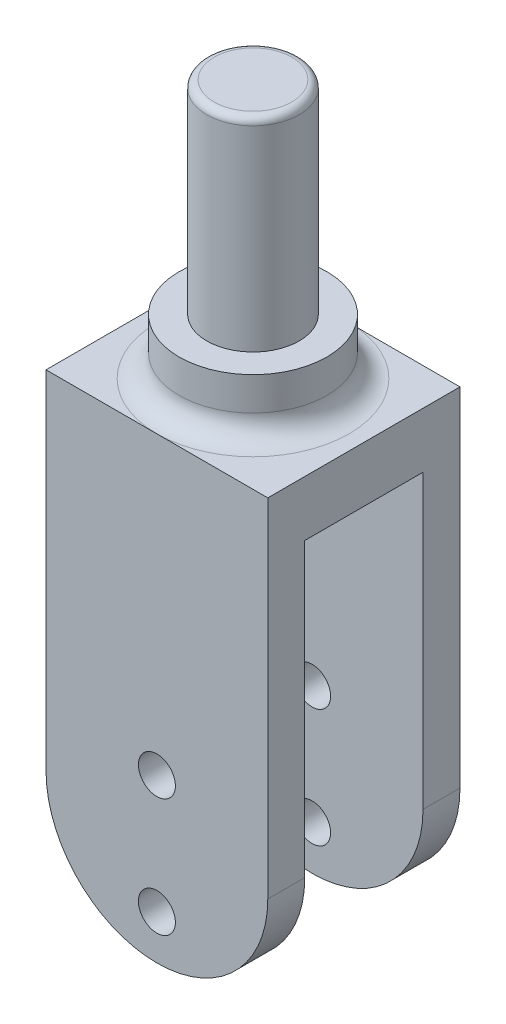
ISO-10303-21;
HEADER;
FILE_DESCRIPTION(('STEP AP214'),'2;1');
FILE_NAME('part.step','',(''),(''),'','','');
FILE_SCHEMA(('AUTOMOTIVE_DESIGN { 1 0 10303 214 1 1 1 1 }'));
ENDSEC;
DATA;
#1=APPLICATION_CONTEXT('core data for automotive mechanical design processes');
#2=APPLICATION_PROTOCOL_DEFINITION('international standard','automotive_design',2000,#1);
#3=PRODUCT_CONTEXT('',#1,'mechanical');
#4=PRODUCT('Part','Part','',(#3));
#5=PRODUCT_RELATED_PRODUCT_CATEGORY('part','',(#4));
#6=PRODUCT_DEFINITION_FORMATION('','',#4);
#7=PRODUCT_DEFINITION_CONTEXT('part definition',#1,'design');
#8=PRODUCT_DEFINITION('design','',#6,#7);
#9=PRODUCT_DEFINITION_SHAPE('','',#8);
#10=(LENGTH_UNIT() NAMED_UNIT(*) SI_UNIT(.MILLI.,.METRE.));
#11=(NAMED_UNIT(*) PLANE_ANGLE_UNIT() SI_UNIT($,.RADIAN.));
#12=(NAMED_UNIT(*) SI_UNIT($,.STERADIAN.) SOLID_ANGLE_UNIT());
#13=UNCERTAINTY_MEASURE_WITH_UNIT(LENGTH_MEASURE(1.E-05),#10,'distance_accuracy_value','');
#14=(GEOMETRIC_REPRESENTATION_CONTEXT(3) GLOBAL_UNCERTAINTY_ASSIGNED_CONTEXT((#13)) GLOBAL_UNIT_ASSIGNED_CONTEXT((#10,
#11,#12)) REPRESENTATION_CONTEXT('',''));
#15=CARTESIAN_POINT('',(0.,0.,0.));
#16=DIRECTION('',(0.,0.,1.));
#17=DIRECTION('',(1.,0.,0.));
#18=AXIS2_PLACEMENT_3D('',#15,#16,#17);
#19=CARTESIAN_POINT('',(0.,-47.,52.));
#20=DIRECTION('',(0.,0.,-1.));
#21=DIRECTION('',(-1.,0.,0.));
#22=AXIS2_PLACEMENT_3D('',#19,#20,#21);
#23=CYLINDRICAL_SURFACE('',#22,30.);
#24=DIRECTION('',(0.,0.,-1.));
#25=VECTOR('',#24,1.);
#26=CARTESIAN_POINT('',(30.,-47.,52.));
#27=LINE('',#26,#25);
#28=CARTESIAN_POINT('',(30.,-47.,9.99999999999999));
#29=VERTEX_POINT('',#28);
#30=CARTESIAN_POINT('',(30.,-47.,0.));
#31=VERTEX_POINT('',#30);
#32=EDGE_CURVE('E154',#29,#31,#27,.T.);
#33=ORIENTED_EDGE('',*,*,#32,.F.);
#34=CARTESIAN_POINT('',(0.,-47.,9.99999999999999));
#35=DIRECTION('',(0.,0.,-1.));
#36=DIRECTION('',(0.,1.,0.));
#37=AXIS2_PLACEMENT_3D('',#34,#35,#36);
#38=CIRCLE('',#37,30.);
#39=CARTESIAN_POINT('',(-30.,-47.,9.99999999999999));
#40=VERTEX_POINT('',#39);
#41=EDGE_CURVE('E202',#29,#40,#38,.T.);
#42=ORIENTED_EDGE('',*,*,#41,.T.);
#43=DIRECTION('',(0.,0.,-1.));
#44=VECTOR('',#43,1.);
#45=CARTESIAN_POINT('',(-30.,-47.,52.));
#46=LINE('',#45,#44);
#47=CARTESIAN_POINT('',(-30.,-47.,0.));
#48=VERTEX_POINT('',#47);
#49=EDGE_CURVE('E135',#40,#48,#46,.T.);
#50=ORIENTED_EDGE('',*,*,#49,.T.);
#51=CARTESIAN_POINT('',(0.,-47.,0.));
#52=DIRECTION('',(0.,0.,1.));
#53=DIRECTION('',(1.,0.,0.));
#54=AXIS2_PLACEMENT_3D('',#51,#52,#53);
#55=CIRCLE('',#54,30.);
#56=EDGE_CURVE('E208',#48,#31,#55,.T.);
#57=ORIENTED_EDGE('',*,*,#56,.T.);
#58=EDGE_LOOP('',(#33,#42,#50,#57));
#59=FACE_BOUND('',#58,.T.);
#60=ADVANCED_FACE('F39',(#59),#23,.T.);
#61=CARTESIAN_POINT('',(-30.,47.,52.));
#62=DIRECTION('',(0.,-1.,0.));
#63=DIRECTION('',(0.,0.,-1.));
#64=AXIS2_PLACEMENT_3D('',#61,#62,#63);
#65=PLANE('',#64);
#66=DIRECTION('',(-1.,0.,0.));
#67=VECTOR('',#66,1.);
#68=CARTESIAN_POINT('',(-30.,47.,52.));
#69=LINE('',#68,#67);
#70=CARTESIAN_POINT('',(0.,47.,52.));
#71=VERTEX_POINT('',#70);
#72=CARTESIAN_POINT('',(-30.,47.,52.));
#73=VERTEX_POINT('',#72);
#74=EDGE_CURVE('E217',#71,#73,#69,.T.);
#75=ORIENTED_EDGE('',*,*,#74,.F.);
#76=CARTESIAN_POINT('',(0.,47.,26.));
#77=DIRECTION('',(0.,-1.,0.));
#78=DIRECTION('',(0.,0.,-1.));
#79=AXIS2_PLACEMENT_3D('',#76,#77,#78);
#80=CIRCLE('',#79,26.);
#81=CARTESIAN_POINT('',(0.,47.,0.));
#82=VERTEX_POINT('',#81);
#83=EDGE_CURVE('E163',#71,#82,#80,.T.);
#84=ORIENTED_EDGE('',*,*,#83,.T.);
#85=DIRECTION('',(-1.,0.,0.));
#86=VECTOR('',#85,1.);
#87=CARTESIAN_POINT('',(-30.,47.,0.));
#88=LINE('',#87,#86);
#89=CARTESIAN_POINT('',(-30.,47.,0.));
#90=VERTEX_POINT('',#89);
#91=EDGE_CURVE('E223',#82,#90,#88,.T.);
#92=ORIENTED_EDGE('',*,*,#91,.T.);
#93=DIRECTION('',(0.,0.,-1.));
#94=VECTOR('',#93,1.);
#95=CARTESIAN_POINT('',(-30.,47.,52.));
#96=LINE('',#95,#94);
#97=EDGE_CURVE('E141',#73,#90,#96,.T.);
#98=ORIENTED_EDGE('',*,*,#97,.F.);
#99=EDGE_LOOP('',(#75,#84,#92,#98));
#100=FACE_BOUND('',#99,.T.);
#101=ADVANCED_FACE('F227',(#100),#65,.F.);
#102=CARTESIAN_POINT('',(-30.,-47.,52.));
#103=VERTEX_POINT('',#102);
#104=CARTESIAN_POINT('',(-30.,-47.,42.));
#105=VERTEX_POINT('',#104);
#106=EDGE_CURVE('E140',#103,#105,#46,.T.);
#107=ORIENTED_EDGE('',*,*,#106,.T.);
#108=CARTESIAN_POINT('',(0.,-47.,42.));
#109=DIRECTION('',(0.,0.,1.));
#110=DIRECTION('',(0.,-1.,0.));
#111=AXIS2_PLACEMENT_3D('',#108,#109,#110);
#112=CIRCLE('',#111,30.);
#113=CARTESIAN_POINT('',(30.,-47.,42.));
#114=VERTEX_POINT('',#113);
#115=EDGE_CURVE('E196',#105,#114,#112,.T.);
#116=ORIENTED_EDGE('',*,*,#115,.T.);
#117=CARTESIAN_POINT('',(30.,-47.,52.));
#118=VERTEX_POINT('',#117);
#119=EDGE_CURVE('E151',#118,#114,#27,.T.);
#120=ORIENTED_EDGE('',*,*,#119,.F.);
#121=CARTESIAN_POINT('',(0.,-47.,52.));
#122=DIRECTION('',(0.,0.,1.));
#123=DIRECTION('',(1.,0.,0.));
#124=AXIS2_PLACEMENT_3D('',#121,#122,#123);
#125=CIRCLE('',#124,30.);
#126=EDGE_CURVE('E214',#103,#118,#125,.T.);
#127=ORIENTED_EDGE('',*,*,#126,.F.);
#128=EDGE_LOOP('',(#107,#116,#120,#127));
#129=FACE_BOUND('',#128,.T.);
#130=ADVANCED_FACE('F245',(#129),#23,.T.);
#131=CARTESIAN_POINT('',(30.,47.,52.));
#132=DIRECTION('',(-1.,0.,0.));
#133=DIRECTION('',(0.,-1.,0.));
#134=AXIS2_PLACEMENT_3D('',#131,#132,#133);
#135=PLANE('',#134);
#136=DIRECTION('',(0.,0.,1.));
#137=VECTOR('',#136,1.);
#138=CARTESIAN_POINT('',(30.,32.,42.));
#139=LINE('',#138,#137);
#140=CARTESIAN_POINT('',(30.,32.,10.));
#141=VERTEX_POINT('',#140);
#142=CARTESIAN_POINT('',(30.,32.,42.));
#143=VERTEX_POINT('',#142);
#144=EDGE_CURVE('E197',#141,#143,#139,.T.);
#145=ORIENTED_EDGE('',*,*,#144,.F.);
#146=DIRECTION('',(0.,1.,0.));
#147=VECTOR('',#146,1.);
#148=CARTESIAN_POINT('',(30.,32.,10.));
#149=LINE('',#148,#147);
#150=EDGE_CURVE('E120',#29,#141,#149,.T.);
#151=ORIENTED_EDGE('',*,*,#150,.F.);
#152=ORIENTED_EDGE('',*,*,#32,.T.);
#153=DIRECTION('',(0.,1.,0.));
#154=VECTOR('',#153,1.);
#155=CARTESIAN_POINT('',(30.,47.,0.));
#156=LINE('',#155,#154);
#157=CARTESIAN_POINT('',(30.,47.,0.));
#158=VERTEX_POINT('',#157);
#159=EDGE_CURVE('E218',#31,#158,#156,.T.);
#160=ORIENTED_EDGE('',*,*,#159,.T.);
#161=DIRECTION('',(0.,0.,-1.));
#162=VECTOR('',#161,1.);
#163=CARTESIAN_POINT('',(30.,47.,52.));
#164=LINE('',#163,#162);
#165=CARTESIAN_POINT('',(30.,47.,52.));
#166=VERTEX_POINT('',#165);
#167=EDGE_CURVE('E147',#166,#158,#164,.T.);
#168=ORIENTED_EDGE('',*,*,#167,.F.);
#169=DIRECTION('',(0.,1.,0.));
#170=VECTOR('',#169,1.);
#171=CARTESIAN_POINT('',(30.,47.,52.));
#172=LINE('',#171,#170);
#173=EDGE_CURVE('E213',#118,#166,#172,.T.);
#174=ORIENTED_EDGE('',*,*,#173,.F.);
#175=ORIENTED_EDGE('',*,*,#119,.T.);
#176=DIRECTION('',(0.,-1.,0.));
#177=VECTOR('',#176,1.);
#178=CARTESIAN_POINT('',(30.,32.,42.));
#179=LINE('',#178,#177);
#180=EDGE_CURVE('E126',#143,#114,#179,.T.);
#181=ORIENTED_EDGE('',*,*,#180,.F.);
#182=EDGE_LOOP('',(#145,#151,#152,#160,#168,#174,#175,#181));
#183=FACE_BOUND('',#182,.T.);
#184=ADVANCED_FACE('F236',(#183),#135,.F.);
#185=EDGE_CURVE('E224',#158,#82,#88,.T.);
#186=ORIENTED_EDGE('',*,*,#185,.T.);
#187=CARTESIAN_POINT('',(0.,47.,26.));
#188=DIRECTION('',(0.,-1.,0.));
#189=DIRECTION('',(0.,0.,-1.));
#190=AXIS2_PLACEMENT_3D('',#187,#188,#189);
#191=CIRCLE('',#190,26.);
#192=EDGE_CURVE('E63',#82,#71,#191,.T.);
#193=ORIENTED_EDGE('',*,*,#192,.T.);
#194=EDGE_CURVE('E144',#166,#71,#69,.T.);
#195=ORIENTED_EDGE('',*,*,#194,.F.);
#196=ORIENTED_EDGE('',*,*,#167,.T.);
#197=EDGE_LOOP('',(#186,#193,#195,#196));
#198=FACE_BOUND('',#197,.T.);
#199=ADVANCED_FACE('F279',(#198),#65,.F.);
#200=CARTESIAN_POINT('',(-30.,47.,52.));
#201=DIRECTION('',(1.,0.,0.));
#202=DIRECTION('',(0.,1.,0.));
#203=AXIS2_PLACEMENT_3D('',#200,#201,#202);
#204=PLANE('',#203);
#205=ORIENTED_EDGE('',*,*,#49,.F.);
#206=DIRECTION('',(0.,1.,0.));
#207=VECTOR('',#206,1.);
#208=CARTESIAN_POINT('',(-30.,47.,10.));
#209=LINE('',#208,#207);
#210=CARTESIAN_POINT('',(-30.,32.,10.));
#211=VERTEX_POINT('',#210);
#212=EDGE_CURVE('E11',#40,#211,#209,.T.);
#213=ORIENTED_EDGE('',*,*,#212,.T.);
#214=DIRECTION('',(0.,0.,1.));
#215=VECTOR('',#214,1.);
#216=CARTESIAN_POINT('',(-30.,32.,42.));
#217=LINE('',#216,#215);
#218=CARTESIAN_POINT('',(-30.,32.,42.));
#219=VERTEX_POINT('',#218);
#220=EDGE_CURVE('E121',#211,#219,#217,.T.);
#221=ORIENTED_EDGE('',*,*,#220,.T.);
#222=DIRECTION('',(0.,-1.,0.));
#223=VECTOR('',#222,1.);
#224=CARTESIAN_POINT('',(-30.,32.,42.));
#225=LINE('',#224,#223);
#226=EDGE_CURVE('E57',#219,#105,#225,.T.);
#227=ORIENTED_EDGE('',*,*,#226,.T.);
#228=ORIENTED_EDGE('',*,*,#106,.F.);
#229=DIRECTION('',(0.,-1.,0.));
#230=VECTOR('',#229,1.);
#231=CARTESIAN_POINT('',(-30.,47.,52.));
#232=LINE('',#231,#230);
#233=EDGE_CURVE('E136',#73,#103,#232,.T.);
#234=ORIENTED_EDGE('',*,*,#233,.F.);
#235=ORIENTED_EDGE('',*,*,#97,.T.);
#236=DIRECTION('',(0.,-1.,0.));
#237=VECTOR('',#236,1.);
#238=CARTESIAN_POINT('',(-30.,47.,0.));
#239=LINE('',#238,#237);
#240=EDGE_CURVE('E133',#90,#48,#239,.T.);
#241=ORIENTED_EDGE('',*,*,#240,.T.);
#242=EDGE_LOOP('',(#205,#213,#221,#227,#228,#234,#235,#241));
#243=FACE_BOUND('',#242,.T.);
#244=ADVANCED_FACE('F127',(#243),#204,.F.);
#245=CARTESIAN_POINT('',(0.,-47.,52.));
#246=DIRECTION('',(0.,0.,1.));
#247=DIRECTION('',(1.,0.,0.));
#248=AXIS2_PLACEMENT_3D('',#245,#246,#247);
#249=PLANE('',#248);
#250=CARTESIAN_POINT('',(0.,-33.,52.));
#251=DIRECTION('',(0.,0.,1.));
#252=DIRECTION('',(1.,0.,0.));
#253=AXIS2_PLACEMENT_3D('',#250,#251,#252);
#254=CIRCLE('',#253,5.);
#255=CARTESIAN_POINT('',(5.,-33.,52.));
#256=VERTEX_POINT('',#255);
#257=EDGE_CURVE('E178',#256,#256,#254,.T.);
#258=ORIENTED_EDGE('',*,*,#257,.F.);
#259=EDGE_LOOP('',(#258));
#260=FACE_BOUND('',#259,.T.);
#261=CARTESIAN_POINT('',(0.,-65.,52.));
#262=DIRECTION('',(0.,0.,1.));
#263=DIRECTION('',(1.,0.,0.));
#264=AXIS2_PLACEMENT_3D('',#261,#262,#263);
#265=CIRCLE('',#264,5.);
#266=CARTESIAN_POINT('',(5.,-65.,52.));
#267=VERTEX_POINT('',#266);
#268=EDGE_CURVE('E189',#267,#267,#265,.T.);
#269=ORIENTED_EDGE('',*,*,#268,.F.);
#270=EDGE_LOOP('',(#269));
#271=FACE_BOUND('',#270,.T.);
#272=ORIENTED_EDGE('',*,*,#126,.T.);
#273=ORIENTED_EDGE('',*,*,#173,.T.);
#274=ORIENTED_EDGE('',*,*,#194,.T.);
#275=ORIENTED_EDGE('',*,*,#74,.T.);
#276=ORIENTED_EDGE('',*,*,#233,.T.);
#277=EDGE_LOOP('',(#272,#273,#274,#275,#276));
#278=FACE_BOUND('',#277,.T.);
#279=ADVANCED_FACE('F244',(#260,#271,#278),#249,.T.);
#280=CARTESIAN_POINT('',(0.,-47.,0.));
#281=DIRECTION('',(0.,0.,1.));
#282=DIRECTION('',(1.,0.,0.));
#283=AXIS2_PLACEMENT_3D('',#280,#281,#282);
#284=PLANE('',#283);
#285=CARTESIAN_POINT('',(0.,-33.,0.));
#286=DIRECTION('',(0.,0.,1.));
#287=DIRECTION('',(1.,0.,0.));
#288=AXIS2_PLACEMENT_3D('',#285,#286,#287);
#289=CIRCLE('',#288,5.);
#290=CARTESIAN_POINT('',(5.,-33.,0.));
#291=VERTEX_POINT('',#290);
#292=EDGE_CURVE('E175',#291,#291,#289,.T.);
#293=ORIENTED_EDGE('',*,*,#292,.T.);
#294=EDGE_LOOP('',(#293));
#295=FACE_BOUND('',#294,.T.);
#296=CARTESIAN_POINT('',(0.,-65.,0.));
#297=DIRECTION('',(0.,0.,1.));
#298=DIRECTION('',(1.,0.,0.));
#299=AXIS2_PLACEMENT_3D('',#296,#297,#298);
#300=CIRCLE('',#299,5.);
#301=CARTESIAN_POINT('',(5.,-65.,0.));
#302=VERTEX_POINT('',#301);
#303=EDGE_CURVE('E182',#302,#302,#300,.T.);
#304=ORIENTED_EDGE('',*,*,#303,.T.);
#305=EDGE_LOOP('',(#304));
#306=FACE_BOUND('',#305,.T.);
#307=ORIENTED_EDGE('',*,*,#56,.F.);
#308=ORIENTED_EDGE('',*,*,#240,.F.);
#309=ORIENTED_EDGE('',*,*,#91,.F.);
#310=ORIENTED_EDGE('',*,*,#185,.F.);
#311=ORIENTED_EDGE('',*,*,#159,.F.);
#312=EDGE_LOOP('',(#307,#308,#309,#310,#311));
#313=FACE_BOUND('',#312,.T.);
#314=ADVANCED_FACE('F235',(#295,#306,#313),#284,.F.);
#315=CARTESIAN_POINT('',(0.,62.,26.));
#316=DIRECTION('',(0.,-1.,0.));
#317=DIRECTION('',(0.,0.,-1.));
#318=AXIS2_PLACEMENT_3D('',#315,#316,#317);
#319=CYLINDRICAL_SURFACE('',#318,20.);
#320=CARTESIAN_POINT('',(0.,53.,26.));
#321=DIRECTION('',(0.,-1.,0.));
#322=DIRECTION('',(0.,0.,-1.));
#323=AXIS2_PLACEMENT_3D('',#320,#321,#322);
#324=CIRCLE('',#323,20.);
#325=CARTESIAN_POINT('',(0.,53.,5.99999999999999));
#326=VERTEX_POINT('',#325);
#327=EDGE_CURVE('E159',#326,#326,#324,.F.);
#328=ORIENTED_EDGE('',*,*,#327,.T.);
#329=EDGE_LOOP('',(#328));
#330=FACE_BOUND('',#329,.T.);
#331=CARTESIAN_POINT('',(0.,62.,26.));
#332=DIRECTION('',(0.,1.,0.));
#333=DIRECTION('',(0.,0.,1.));
#334=AXIS2_PLACEMENT_3D('',#331,#332,#333);
#335=CIRCLE('',#334,20.);
#336=CARTESIAN_POINT('',(0.,62.,46.));
#337=VERTEX_POINT('',#336);
#338=EDGE_CURVE('E201',#337,#337,#335,.T.);
#339=ORIENTED_EDGE('',*,*,#338,.F.);
#340=EDGE_LOOP('',(#339));
#341=FACE_BOUND('',#340,.T.);
#342=ADVANCED_FACE('F251',(#330,#341),#319,.T.);
#343=CARTESIAN_POINT('',(0.,62.,26.));
#344=DIRECTION('',(0.,1.,0.));
#345=DIRECTION('',(0.,0.,1.));
#346=AXIS2_PLACEMENT_3D('',#343,#344,#345);
#347=PLANE('',#346);
#348=CARTESIAN_POINT('',(0.,62.,26.));
#349=DIRECTION('',(0.,1.,0.));
#350=DIRECTION('',(0.,0.,1.));
#351=AXIS2_PLACEMENT_3D('',#348,#349,#350);
#352=CIRCLE('',#351,12.5);
#353=CARTESIAN_POINT('',(0.,62.,38.5));
#354=VERTEX_POINT('',#353);
#355=EDGE_CURVE('E165',#354,#354,#352,.T.);
#356=ORIENTED_EDGE('',*,*,#355,.F.);
#357=EDGE_LOOP('',(#356));
#358=FACE_BOUND('',#357,.T.);
#359=ORIENTED_EDGE('',*,*,#338,.T.);
#360=EDGE_LOOP('',(#359));
#361=FACE_BOUND('',#360,.T.);
#362=ADVANCED_FACE('F252',(#358,#361),#347,.T.);
#363=CARTESIAN_POINT('',(0.,53.,26.));
#364=DIRECTION('',(0.,-1.,0.));
#365=DIRECTION('',(0.,0.,-1.));
#366=AXIS2_PLACEMENT_3D('',#363,#364,#365);
#367=TOROIDAL_SURFACE('',#366,26.,6.);
#368=ORIENTED_EDGE('',*,*,#192,.F.);
#369=ORIENTED_EDGE('',*,*,#83,.F.);
#370=EDGE_LOOP('',(#368,#369));
#371=FACE_BOUND('',#370,.T.);
#372=ORIENTED_EDGE('',*,*,#327,.F.);
#373=EDGE_LOOP('',(#372));
#374=FACE_BOUND('',#373,.T.);
#375=ADVANCED_FACE('F250',(#371,#374),#367,.F.);
#376=CARTESIAN_POINT('',(0.,117.,26.));
#377=DIRECTION('',(0.,-1.,0.));
#378=DIRECTION('',(0.,0.,-1.));
#379=AXIS2_PLACEMENT_3D('',#376,#377,#378);
#380=CYLINDRICAL_SURFACE('',#379,12.5);
#381=CARTESIAN_POINT('',(0.,115.,26.));
#382=DIRECTION('',(0.,1.,0.));
#383=DIRECTION('',(0.,0.,1.));
#384=AXIS2_PLACEMENT_3D('',#381,#382,#383);
#385=CIRCLE('',#384,12.5);
#386=CARTESIAN_POINT('',(0.,115.,38.5));
#387=VERTEX_POINT('',#386);
#388=EDGE_CURVE('E48',#387,#387,#385,.F.);
#389=ORIENTED_EDGE('',*,*,#388,.T.);
#390=EDGE_LOOP('',(#389));
#391=FACE_BOUND('',#390,.T.);
#392=ORIENTED_EDGE('',*,*,#355,.T.);
#393=EDGE_LOOP('',(#392));
#394=FACE_BOUND('',#393,.T.);
#395=ADVANCED_FACE('F249',(#391,#394),#380,.T.);
#396=CARTESIAN_POINT('',(0.,117.,26.));
#397=DIRECTION('',(0.,1.,0.));
#398=DIRECTION('',(0.,0.,1.));
#399=AXIS2_PLACEMENT_3D('',#396,#397,#398);
#400=PLANE('',#399);
#401=CARTESIAN_POINT('',(0.,117.,26.));
#402=DIRECTION('',(0.,1.,0.));
#403=DIRECTION('',(0.,0.,1.));
#404=AXIS2_PLACEMENT_3D('',#401,#402,#403);
#405=CIRCLE('',#404,10.5);
#406=CARTESIAN_POINT('',(0.,117.,36.5));
#407=VERTEX_POINT('',#406);
#408=EDGE_CURVE('E164',#407,#407,#405,.T.);
#409=ORIENTED_EDGE('',*,*,#408,.T.);
#410=EDGE_LOOP('',(#409));
#411=FACE_BOUND('',#410,.T.);
#412=ADVANCED_FACE('F326',(#411),#400,.T.);
#413=CARTESIAN_POINT('',(0.,115.,26.));
#414=DIRECTION('',(0.,1.,0.));
#415=DIRECTION('',(0.,0.,1.));
#416=AXIS2_PLACEMENT_3D('',#413,#414,#415);
#417=TOROIDAL_SURFACE('',#416,10.5,2.);
#418=ORIENTED_EDGE('',*,*,#388,.F.);
#419=EDGE_LOOP('',(#418));
#420=FACE_BOUND('',#419,.T.);
#421=ORIENTED_EDGE('',*,*,#408,.F.);
#422=EDGE_LOOP('',(#421));
#423=FACE_BOUND('',#422,.T.);
#424=ADVANCED_FACE('F41',(#420,#423),#417,.T.);
#425=CARTESIAN_POINT('',(-30.,32.,10.));
#426=DIRECTION('',(0.,0.,-1.));
#427=DIRECTION('',(0.,1.,0.));
#428=AXIS2_PLACEMENT_3D('',#425,#426,#427);
#429=PLANE('',#428);
#430=CARTESIAN_POINT('',(0.,-33.,9.99999999999999));
#431=DIRECTION('',(0.,0.,-1.));
#432=DIRECTION('',(0.,1.,0.));
#433=AXIS2_PLACEMENT_3D('',#430,#431,#432);
#434=CIRCLE('',#433,5.);
#435=CARTESIAN_POINT('',(0.,-28.,9.99999999999999));
#436=VERTEX_POINT('',#435);
#437=EDGE_CURVE('E194',#436,#436,#434,.T.);
#438=ORIENTED_EDGE('',*,*,#437,.T.);
#439=EDGE_LOOP('',(#438));
#440=FACE_BOUND('',#439,.T.);
#441=CARTESIAN_POINT('',(0.,-65.,9.99999999999999));
#442=DIRECTION('',(0.,0.,-1.));
#443=DIRECTION('',(0.,1.,0.));
#444=AXIS2_PLACEMENT_3D('',#441,#442,#443);
#445=CIRCLE('',#444,5.);
#446=CARTESIAN_POINT('',(0.,-60.,9.99999999999999));
#447=VERTEX_POINT('',#446);
#448=EDGE_CURVE('E171',#447,#447,#445,.T.);
#449=ORIENTED_EDGE('',*,*,#448,.T.);
#450=EDGE_LOOP('',(#449));
#451=FACE_BOUND('',#450,.T.);
#452=ORIENTED_EDGE('',*,*,#150,.T.);
#453=DIRECTION('',(1.,0.,0.));
#454=VECTOR('',#453,1.);
#455=CARTESIAN_POINT('',(-30.,32.,10.));
#456=LINE('',#455,#454);
#457=EDGE_CURVE('E115',#211,#141,#456,.T.);
#458=ORIENTED_EDGE('',*,*,#457,.F.);
#459=ORIENTED_EDGE('',*,*,#212,.F.);
#460=ORIENTED_EDGE('',*,*,#41,.F.);
#461=EDGE_LOOP('',(#452,#458,#459,#460));
#462=FACE_BOUND('',#461,.T.);
#463=ADVANCED_FACE('F112',(#440,#451,#462),#429,.F.);
#464=CARTESIAN_POINT('',(-30.,32.,42.));
#465=DIRECTION('',(0.,0.,1.));
#466=DIRECTION('',(0.,-1.,0.));
#467=AXIS2_PLACEMENT_3D('',#464,#465,#466);
#468=PLANE('',#467);
#469=CARTESIAN_POINT('',(0.,-33.,42.));
#470=DIRECTION('',(0.,0.,1.));
#471=DIRECTION('',(0.,-1.,0.));
#472=AXIS2_PLACEMENT_3D('',#469,#470,#471);
#473=CIRCLE('',#472,5.);
#474=CARTESIAN_POINT('',(0.,-38.,42.));
#475=VERTEX_POINT('',#474);
#476=EDGE_CURVE('E43',#475,#475,#473,.T.);
#477=ORIENTED_EDGE('',*,*,#476,.T.);
#478=EDGE_LOOP('',(#477));
#479=FACE_BOUND('',#478,.T.);
#480=CARTESIAN_POINT('',(0.,-65.,42.));
#481=DIRECTION('',(0.,0.,1.));
#482=DIRECTION('',(0.,-1.,0.));
#483=AXIS2_PLACEMENT_3D('',#480,#481,#482);
#484=CIRCLE('',#483,5.);
#485=CARTESIAN_POINT('',(0.,-70.,42.));
#486=VERTEX_POINT('',#485);
#487=EDGE_CURVE('E169',#486,#486,#484,.T.);
#488=ORIENTED_EDGE('',*,*,#487,.T.);
#489=EDGE_LOOP('',(#488));
#490=FACE_BOUND('',#489,.T.);
#491=ORIENTED_EDGE('',*,*,#226,.F.);
#492=DIRECTION('',(1.,0.,0.));
#493=VECTOR('',#492,1.);
#494=CARTESIAN_POINT('',(-30.,32.,42.));
#495=LINE('',#494,#493);
#496=EDGE_CURVE('E122',#219,#143,#495,.T.);
#497=ORIENTED_EDGE('',*,*,#496,.T.);
#498=ORIENTED_EDGE('',*,*,#180,.T.);
#499=ORIENTED_EDGE('',*,*,#115,.F.);
#500=EDGE_LOOP('',(#491,#497,#498,#499));
#501=FACE_BOUND('',#500,.T.);
#502=ADVANCED_FACE('F239',(#479,#490,#501),#468,.F.);
#503=CARTESIAN_POINT('',(-30.,32.,42.));
#504=DIRECTION('',(0.,1.,0.));
#505=DIRECTION('',(-1.,0.,0.));
#506=AXIS2_PLACEMENT_3D('',#503,#504,#505);
#507=PLANE('',#506);
#508=ORIENTED_EDGE('',*,*,#144,.T.);
#509=ORIENTED_EDGE('',*,*,#496,.F.);
#510=ORIENTED_EDGE('',*,*,#220,.F.);
#511=ORIENTED_EDGE('',*,*,#457,.T.);
#512=EDGE_LOOP('',(#508,#509,#510,#511));
#513=FACE_BOUND('',#512,.T.);
#514=ADVANCED_FACE('F123',(#513),#507,.F.);
#515=CARTESIAN_POINT('',(0.,-65.,0.));
#516=DIRECTION('',(0.,0.,1.));
#517=DIRECTION('',(1.,0.,0.));
#518=AXIS2_PLACEMENT_3D('',#515,#516,#517);
#519=CYLINDRICAL_SURFACE('',#518,5.);
#520=ORIENTED_EDGE('',*,*,#268,.T.);
#521=EDGE_LOOP('',(#520));
#522=FACE_BOUND('',#521,.T.);
#523=ORIENTED_EDGE('',*,*,#487,.F.);
#524=EDGE_LOOP('',(#523));
#525=FACE_BOUND('',#524,.T.);
#526=ADVANCED_FACE('F296',(#522,#525),#519,.F.);
#527=CARTESIAN_POINT('',(0.,-33.,0.));
#528=DIRECTION('',(0.,0.,1.));
#529=DIRECTION('',(1.,0.,0.));
#530=AXIS2_PLACEMENT_3D('',#527,#528,#529);
#531=CYLINDRICAL_SURFACE('',#530,5.);
#532=ORIENTED_EDGE('',*,*,#257,.T.);
#533=EDGE_LOOP('',(#532));
#534=FACE_BOUND('',#533,.T.);
#535=ORIENTED_EDGE('',*,*,#476,.F.);
#536=EDGE_LOOP('',(#535));
#537=FACE_BOUND('',#536,.T.);
#538=ADVANCED_FACE('F301',(#534,#537),#531,.F.);
#539=ORIENTED_EDGE('',*,*,#303,.F.);
#540=EDGE_LOOP('',(#539));
#541=FACE_BOUND('',#540,.T.);
#542=ORIENTED_EDGE('',*,*,#448,.F.);
#543=EDGE_LOOP('',(#542));
#544=FACE_BOUND('',#543,.T.);
#545=ADVANCED_FACE('F303',(#541,#544),#519,.F.);
#546=ORIENTED_EDGE('',*,*,#292,.F.);
#547=EDGE_LOOP('',(#546));
#548=FACE_BOUND('',#547,.T.);
#549=ORIENTED_EDGE('',*,*,#437,.F.);
#550=EDGE_LOOP('',(#549));
#551=FACE_BOUND('',#550,.T.);
#552=ADVANCED_FACE('F309',(#548,#551),#531,.F.);
#553=CLOSED_SHELL('',(#60,#101,#130,#184,#199,#244,#279,#314,#342,#362,#375,#395,#412,#424,#463,
#502,#514,#526,#538,#545,#552));
#554=MANIFOLD_SOLID_BREP('B2',#553);
#555=ADVANCED_BREP_SHAPE_REPRESENTATION('',(#18,#554),#14);
#556=SHAPE_DEFINITION_REPRESENTATION(#9,#555);
ENDSEC;
END-ISO-10303-21;
